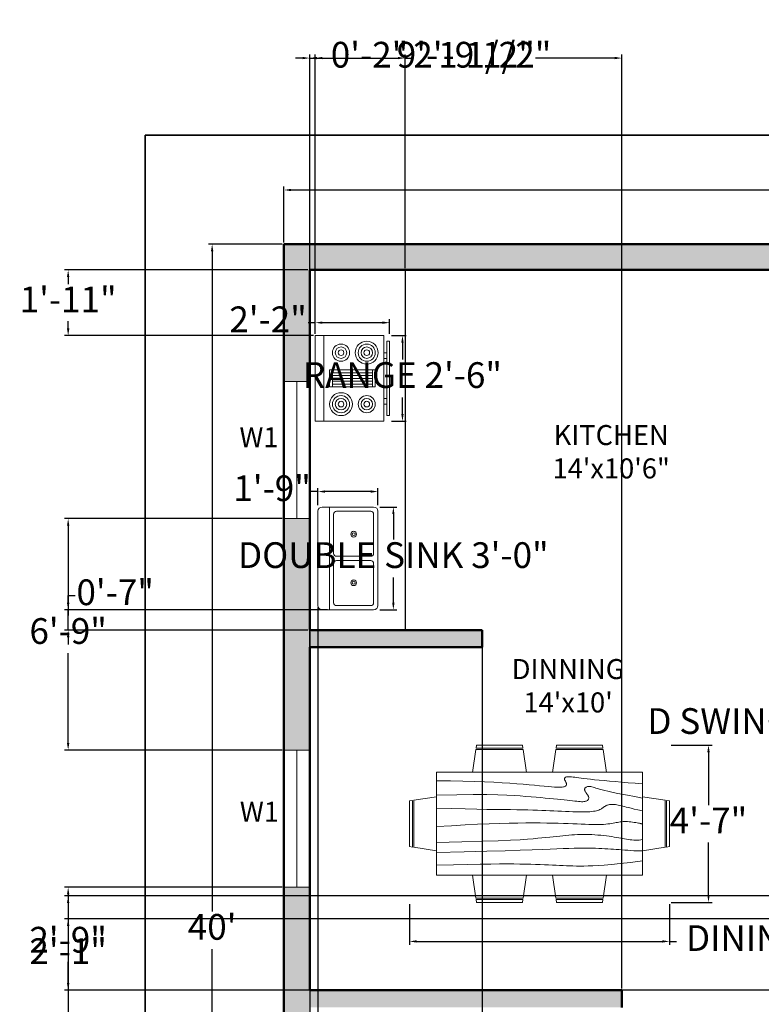
# Model space of a CAD drawing. Units: inches. Extents: x 6193 to 6719, y 6945 to 7563.
# Tile 3 of 4: x 6200 to 6459, y 7219 to 7563. Entities that reach past the tile are written whole.
import ezdxf

# ---------------------------------------------------------------- set-up
doc = ezdxf.new("R2010")
doc.units = ezdxf.units.IN
for name, color, linetype, lineweight in [('A-ANNO-DIMS', 2, 'Continuous', 18), ('A-ANNO-TEXT', 7, 'Continuous', 18), ('A-ANNO-TTLB', 7, 'Continuous', 35), ('A-AREA-IDEN', 7, 'Continuous', 25), ('A-EQPM', 8, 'Continuous', 18), ('A-FLOR-CASE', 8, 'Continuous', 25), ('A-FLOR-FIXT', 9, 'Continuous', 18), ('A-FURN', 8, 'Continuous', 18), ('A-GLAZ', 4, 'Continuous', 18), ('A-WALL', 7, 'Continuous', 50)]:
    doc.layers.add(name, color=color, linetype=linetype, lineweight=lineweight)
doc.layers.add('A-WALL-PATT', color=18, linetype='Continuous', lineweight=13, true_color=0x000000)
doc.styles.get("Standard").update_dxf_attribs({"font": 'arial.ttf'})
doc.dimstyles.new('ISO-25', dxfattribs={"dimtxt": 9, "dimasz": 2.5, "dimexe": 1.25, "dimexo": 0.625, "dimgap": 2, "dimtad": 0, "dimtih": 1, "dimtoh": 1, "dimdec": 1, "dimlunit": 4, "dimtxsty": 'Standard', "dimcen": 2.5, "dimadec": 0, "dimazin": 0, "dimtfac": 0.5, "dimtdec": 1, "dimtmove": 0, "dimatfit": 3, "dimfxl": 1, "dimarcsym": 0})

# ---------------------------------------------------------------- blocks, each defined once
blk = doc.blocks.new('Dining Set - 36 x 72 in.')
for p, q in [((-22.2343, 26.00059), (-23.4847, 17.99762)), ((-22.2304, 26), (-5.7608, 26)), ((-22, 27.5), (-22.1562, 26.50042)), ((-5.8416, 26.5), (-22.1534, 26.5)), ((-22, 27.5), (-6, 27.5)), ((-5.8437, 26.49966), (-6, 27.5)), ((-4.5152, 17.99762), (-5.7655, 25.99926)), ((5.7657, 26.00059), (4.5153, 17.99762)), ((5.7696, 26), (22.2392, 26)), ((6, 27.5), (5.8438, 26.50042)), ((22.1584, 26.5), (5.8466, 26.5)), ((6, 27.5), (22, 27.5)), ((22.1563, 26.49966), (22, 27.5)), ((23.4848, 17.99762), (22.2345, 25.99926)), ((36, 18), (-36, 18)), ((-36, 18), (-36, -18)), ((36, -18), (36, 18)), ((-45.5, 8), (-44.5004, 8.15617)), ((-45.5, 8), (-45.5, -8)), ((-44.5, -8.15843), (-44.5, 8.15338)), ((-44.0006, 8.23428), (-35.9976, 9.48474)), ((-44, 8.23041), (-44, -8.23915)), ((44.0006, 8.23428), (35.9976, 9.48474)), ((44, 8.23041), (44, -8.23915)), ((44.5, -8.15843), (44.5, 8.15338)), ((45.5, 8), (44.5005, 8.15617)), ((45.5, 8), (45.5, -8)), ((-44.4997, -8.15631), (-45.5, -8)), ((-35.9976, -9.48476), (-43.9993, -8.2345)), ((35.9976, -9.48476), (43.9993, -8.2345)), ((44.4997, -8.15631), (45.5, -8)), ((-36, -18), (36, -18)), ((-22.2343, -26.0006), (-23.4847, -17.99762)), ((-4.5152, -17.99762), (-5.7655, -25.99928)), ((5.7657, -26.0006), (4.5153, -17.99762)), ((23.4848, -17.99762), (22.2345, -25.99928)), ((-22.2304, -26), (-5.7608, -26)), ((-22, -27.5), (-22.1562, -26.50044)), ((-5.8416, -26.5), (-22.1534, -26.5)), ((-22, -27.5), (-6, -27.5)), ((-5.8437, -26.49967), (-6, -27.5)), ((5.7696, -26), (22.2392, -26)), ((6, -27.5), (5.8438, -26.50044)), ((22.1584, -26.5), (5.8466, -26.5)), ((6, -27.5), (22, -27.5)), ((22.1563, -26.49967), (22, -27.5))]:
    blk.add_line(p, q)
for points in [[(-36, 15), (-31.1772, 14.97754), (-26.8079, 14.91406), (-22.8538, 14.81543), (-19.276, 14.6875), (-16.0362, 14.53613), (-13.0957, 14.36718), (-10.4159, 14.18652), (-7.9583, 14), (-5.6904, 13.81315), (-3.6035, 13.63021), (-1.6954, 13.45508), (0.0365, 13.29166), (1.5945, 13.14388), (2.9811, 13.01562), (4.1988, 12.9108), (5.25, 12.83333), (6.1393, 12.78613), (6.8802, 12.76823), (7.4883, 12.77767), (7.9792, 12.8125), (8.3685, 12.87077), (8.6719, 12.95052), (8.9049, 13.0498), (9.0833, 13.16666), (9.2205, 13.29899), (9.3216, 13.44401), (9.3895, 13.59879), (9.4271, 13.76041), (9.4373, 13.92594), (9.4232, 14.09245), (9.3875, 14.257), (9.3333, 14.41666), (9.2638, 14.56917), (9.1836, 14.71484), (9.0975, 14.85465), (9.0104, 14.98958), (8.9272, 15.1206), (8.8529, 15.2487), (8.7922, 15.37483), (8.75, 15.5), (8.7305, 15.62467), (8.7344, 15.74739), (8.7617, 15.86621), (8.8125, 15.97916), (8.8867, 16.08431), (8.9844, 16.17968), (9.1055, 16.26334), (9.25, 16.33333), (9.4189, 16.38802), (9.6172, 16.42708), (9.8506, 16.45052), (10.125, 16.45833), (10.4463, 16.45052), (10.8203, 16.42708), (11.2529, 16.38802), (11.75, 16.33333), (12.3184, 16.26318), (12.9694, 16.17838), (13.7151, 16.07991), (14.5677, 15.96875), (15.5395, 15.84586), (16.6426, 15.71224), (17.8893, 15.56884), (19.2917, 15.41666), (20.859, 15.25667), (22.5879, 15.08984), (24.4721, 14.91715), (26.5052, 14.73958), (28.6809, 14.5581), (30.9929, 14.3737), (33.4347, 14.18733), (36, 14)], [(-36, 10), (-28.9766, 10.14274), (-23.1725, 10.20442), (-18.4241, 10.19775), (-14.5677, 10.13541), (-11.4399, 10.03011), (-8.877, 9.89453), (-6.7154, 9.74137), (-4.7917, 9.58333), (-2.9698, 9.43082), (-1.2246, 9.28515), (0.4415, 9.14534), (2.026, 9.01041), (3.5266, 8.87939), (4.9408, 8.7513), (6.266, 8.62516), (7.5, 8.5), (8.6411, 8.37549), (9.6914, 8.2539), (10.6538, 8.13818), (11.5312, 8.03125), (12.3267, 7.93603), (13.043, 7.85547), (13.6831, 7.79248), (14.25, 7.75), (14.7471, 7.7303), (15.1797, 7.73307), (15.5537, 7.75732), (15.875, 7.80208), (16.1494, 7.86637), (16.3828, 7.94922), (16.5811, 8.04964), (16.75, 8.16666), (16.8944, 8.29915), (17.0143, 8.44531), (17.1089, 8.60319), (17.1771, 8.77083), (17.218, 8.94629), (17.2305, 9.1276), (17.2137, 9.31282), (17.1667, 9.5), (17.0895, 9.6875), (16.987, 9.875), (16.8649, 10.0625), (16.7292, 10.25), (16.5856, 10.4375), (16.4401, 10.625), (16.2985, 10.8125), (16.1667, 11), (16.05, 11.18733), (15.9518, 11.3737), (15.8752, 11.5581), (15.8229, 11.73958), (15.798, 11.91715), (15.8034, 12.08984), (15.842, 12.25667), (15.9167, 12.41666), (16.0295, 12.56836), (16.1784, 12.70833), (16.3605, 12.83268), (16.5729, 12.9375), (16.8127, 13.01888), (17.0768, 13.07291), (17.3625, 13.0957), (17.6667, 13.08333), (17.9894, 13.03312), (18.3418, 12.94726), (18.7382, 12.82918), (19.1927, 12.68229), (19.7195, 12.51001), (20.3327, 12.31575), (21.0465, 12.10294), (21.875, 11.875), (22.8357, 11.63354), (23.959, 11.37304), (25.2786, 11.08618), (26.8282, 10.76562), (28.6414, 10.40405), (30.752, 9.99414), (33.1936, 9.52856), (36, 9)], [(-36, 5.5), (-30.7157, 5.3348), (-26.069, 5.20963), (-21.9946, 5.11767), (-18.4271, 5.05208), (-15.3009, 5.00602), (-12.5508, 4.97265), (-10.1112, 4.94515), (-7.9167, 4.91666), (-5.909, 4.88167), (-4.0586, 4.83984), (-2.3429, 4.79215), (-0.7396, 4.73958), (0.7739, 4.6831), (2.22, 4.6237), (3.6213, 4.56233), (5, 4.5), (6.373, 4.43782), (7.7344, 4.3776), (9.0723, 4.32129), (10.375, 4.27083), (11.6309, 4.22819), (12.8281, 4.19531), (13.9551, 4.17415), (15, 4.16666), (15.954, 4.17448), (16.819, 4.19791), (17.6001, 4.23698), (18.3021, 4.29166), (18.9299, 4.36198), (19.4883, 4.44791), (19.9823, 4.54948), (20.4167, 4.66666), (20.7969, 4.79899), (21.1302, 4.94401), (21.4245, 5.09879), (21.6875, 5.26041), (21.9271, 5.42594), (22.1511, 5.59245), (22.3672, 5.757), (22.5834, 5.91666), (22.8065, 6.06868), (23.0404, 6.21093), (23.2879, 6.34147), (23.5521, 6.45833), (23.8358, 6.55957), (24.142, 6.64323), (24.4735, 6.70735), (24.8334, 6.75), (25.2235, 6.76969), (25.642, 6.76692), (26.0858, 6.74267), (26.5521, 6.69791), (27.0379, 6.63362), (27.5404, 6.55078), (28.0565, 6.45036), (28.5834, 6.33333), (29.1242, 6.19987), (29.7071, 6.04687), (30.3661, 5.87044), (31.1354, 5.66666), (32.0493, 5.43164), (33.142, 5.16146), (34.4475, 4.85221), (36, 4.5)], [(-36, -1), (-30.7915, -0.6591), (-26.0195, -0.38216), (-21.6519, -0.16284), (-17.6563, 0.00521), (-14.0005, 0.12833), (-10.6523, 0.21289), (-7.5796, 0.26522), (-4.75, 0.29166), (-2.134, 0.29793), (0.2878, 0.28711), (2.5317, 0.26163), (4.6146, 0.22396), (6.5529, 0.17651), (8.3633, 0.12174), (10.0623, 0.06209), (11.6667, 0), (13.1899, -0.06201), (14.6341, -0.1211), (15.9982, -0.17432), (17.2813, -0.21875), (18.4823, -0.25147), (19.6003, -0.26953), (20.6343, -0.27002), (21.5834, -0.25), (22.4481, -0.20768), (23.2357, -0.14584), (23.9549, -0.06836), (24.6146, 0.02083), (25.2235, 0.11784), (25.7904, 0.21875), (26.3241, 0.31966), (26.8334, 0.41666), (27.3265, 0.50618), (27.8099, 0.58593), (28.2894, 0.65397), (28.7709, 0.70833), (29.2601, 0.74707), (29.763, 0.76823), (30.2855, 0.76985), (30.8334, 0.75), (31.4088, 0.70784), (31.9994, 0.64713), (32.589, 0.57275), (33.1615, 0.48958), (33.7008, 0.4025), (34.1908, 0.3164), (34.6153, 0.23616), (34.9584, 0.16666), (35.2099, 0.11165), (35.3848, 0.07031), (35.504, 0.04069), (35.5886, 0.02083), (35.6594, 0.00879), (35.7377, 0.0026), (35.8442, 0.00032), (36, 0)], [(-36, -6.5), (-27.1843, -6.31267), (-20.084, -6.1263), (-14.469, -5.9419), (-10.1094, -5.76042), (-6.7752, -5.58285), (-4.2363, -5.41016), (-2.2629, -5.24333), (-0.625, -5.08334), (0.8708, -4.93099), (2.2715, -4.78646), (3.5872, -4.64974), (4.8281, -4.52084), (6.0046, -4.39974), (7.127, -4.28646), (8.2053, -4.18099), (9.25, -4.08334), (10.2705, -3.99382), (11.2734, -3.91407), (12.2647, -3.84603), (13.25, -3.79167), (14.2354, -3.75293), (15.2266, -3.73177), (16.2295, -3.73015), (17.25, -3.75), (18.2912, -3.79248), (19.3451, -3.85547), (20.4009, -3.93604), (21.4479, -4.03125), (22.4754, -4.13819), (23.4727, -4.25391), (24.4289, -4.37549), (25.3334, -4.5), (26.1785, -4.62492), (26.9694, -4.74935), (27.7145, -4.87281), (28.4219, -4.99479), (29.1, -5.11483), (29.7572, -5.23242), (30.4016, -5.34709), (31.0417, -5.45834), (31.6837, -5.56437), (32.3262, -5.65821), (32.9658, -5.73153), (33.599, -5.77604), (34.2224, -5.78345), (34.8327, -5.74545), (35.4264, -5.65373), (36, -5.5)], [(-36, -10), (-26.4022, -9.81299), (-18.4675, -9.62891), (-11.9839, -9.45069), (-6.7396, -9.28125), (-2.5226, -9.12354), (0.8789, -8.98047), (3.6769, -8.85498), (6.0833, -8.75), (8.2767, -8.66765), (10.3021, -8.60677), (12.1712, -8.56543), (13.8958, -8.54167), (15.4876, -8.53353), (16.9583, -8.53907), (18.3197, -8.55632), (19.5834, -8.58334), (20.7616, -8.61841), (21.8685, -8.66081), (22.9188, -8.71004), (23.9271, -8.76563), (24.9081, -8.82707), (25.8763, -8.89388), (26.8465, -8.96558), (27.8334, -9.04167), (28.8474, -9.12118), (29.8828, -9.20117), (30.93, -9.27824), (31.9792, -9.34896), (33.0205, -9.40991), (34.0443, -9.45768), (35.0407, -9.48885), (36, -9.5)], [(-36, -14.5), (-30.0881, -14.33513), (-25.0332, -14.21224), (-20.7312, -14.12647), (-17.0781, -14.07292), (-13.97, -14.04671), (-11.3027, -14.04297), (-8.9724, -14.05681), (-6.875, -14.08334), (-4.9224, -14.11833), (-3.0905, -14.16016), (-1.3709, -14.20785), (0.2448, -14.26042), (1.7647, -14.3169), (3.1973, -14.3763), (4.5507, -14.43767), (5.8333, -14.5), (7.0554, -14.5621), (8.235, -14.62175), (9.3922, -14.67652), (10.5469, -14.72396), (11.7192, -14.76164), (12.929, -14.78711), (14.1965, -14.79794), (15.5417, -14.79167), (16.9933, -14.76424), (18.6152, -14.70508), (20.4804, -14.60197), (22.6615, -14.44271), (25.2312, -14.21509), (28.2624, -13.9069), (31.8277, -13.50594), (36, -13)]]:
    blk.add_lwpolyline(points)
blk = doc.blocks.new('Range-Oven - 30 in top')
for p, q in [((0, -3), (30, -3)), ((12, -6), (18, -6)), ((13, -20), (13, -6)), ((14, -6), (14, -20)), ((15, -20), (15, -6)), ((16, -6), (16, -20)), ((17, -20), (17, -6)), ((18, -20), (12, -20)), ((6, -24), (6, -25)), ((8, -25), (8, -24)), ((22, -25), (22, -24)), ((24, -24), (24, -25))]:
    blk.add_line(p, q)
for points in [[(0, -24), (0, 0), (30, 0), (30, -24)], [(12, -21), (12, -5), (18, -5), (18, -21)], [(2, -26), (2, -25), (28, -25), (28, -26)]]:
    blk.add_lwpolyline(points, close=True)
for centre, radius in [((6, -9), 4), ((6, -9), 3), ((24, -9), 3), ((6, -9), 2), ((6, -9), 1), ((24, -9), 2), ((24, -9), 1), ((6, -18), 3), ((6, -18), 2), ((6, -18), 1), ((24, -18), 4), ((24, -18), 3), ((24, -18), 2), ((24, -18), 1)]:
    blk.add_circle(centre, radius)
blk = doc.blocks.new('Sink-double - 36 in top')
for p, q in [((-18, -4), (18, -4)), ((-0.75, -18.5), (-0.75, -6.5)), ((0.75, -6.5), (0.75, -18.5))]:
    blk.add_line(p, q)
for points in [[(-16.5, 0), (16.5, 0)], [(-18, -19.5), (-18, -1.5)], [(18, -1.5), (18, -19.5)], [(-16.5, -18.5), (-16.5, -6.5)], [(-15.5, -5.5), (-1.75, -5.5)], [(1.75, -5.5), (15.5, -5.5)], [(16.5, -6.5), (16.5, -18.5)], [(-1.75, -19.5), (-15.5, -19.5)], [(15.5, -19.5), (1.75, -19.5)], [(16.5, -21), (-16.5, -21)]]:
    blk.add_lwpolyline(points)
for centre, radius in [((-8.5, -12.5), 1), ((-8.5, -12.5), 0.5), ((8.5, -12.5), 1), ((8.5, -12.5), 0.5)]:
    blk.add_circle(centre, radius)
for centre, radius, start, end in [((-16.5, -1.5), 1.5, 90, 180), ((16.5, -1.5), 1.5, 0, 90), ((-15.5, -6.5), 1, 90, 180), ((-1.75, -6.5), 1, 0, 90), ((1.75, -6.5), 1, 90, 180), ((15.5, -6.5), 1, 0, 90), ((-16.5, -19.5), 1.5, 180, 270), ((-15.5, -18.5), 1, 180, 270), ((-1.75, -18.5), 1, 270, 0), ((1.75, -18.5), 1, 180, 270), ((15.5, -18.5), 1, 270, 0), ((16.5, -19.5), 1.5, 270, 0)]:
    blk.add_arc(centre, radius, start, end)
blk = doc.blocks.new('*D10')
at = {"layer": 'A-ANNO-DIMS', "color": 0, "lineweight": -2, "transparency": 16777216}
for p, q in [((6292.28, 7485.29), (6292.28, 7504.87)), ((6294.78, 7503.62), (6462.65, 7503.62)), ((6649.78, 7503.62), (6481.92, 7503.62)), ((6652.28, 7485.29), (6652.28, 7504.87))]:
    blk.add_line(p, q, dxfattribs=at)
at = {"layer": 'A-ANNO-DIMS', "color": 0, "transparency": 16777216}
for points in [[(6294.78, 7504.03), (6294.78, 7503.2), (6292.28, 7503.62)], [(6649.78, 7504.03), (6649.78, 7503.2), (6652.28, 7503.62)]]:
    blk.add_solid(points, dxfattribs=at)
at = {"layer": 'Defpoints', "color": 0, "transparency": 16777216}
for p in [(6652.28, 7503.62), (6292.28, 7484.66), (6652.28, 7484.66)]:
    blk.add_point(p, dxfattribs=at)
at = {"layer": 'A-ANNO-DIMS', "color": 0, "transparency": 16777216, "insert": (6472.28, 7503.62), "char_height": 9, "attachment_point": 5}
blk.add_mtext("30'", dxfattribs=at)
blk = doc.blocks.new('*D11')
at = {"layer": 'A-ANNO-DIMS', "color": 0, "lineweight": -2, "transparency": 16777216}
for p, q in [((6291.66, 7484.66), (6265.88, 7484.66)), ((6267.13, 7482.16), (6267.13, 7251.26)), ((6267.13, 7007.16), (6267.13, 7238.07)), ((6291.66, 7004.66), (6265.88, 7004.66))]:
    blk.add_line(p, q, dxfattribs=at)
at = {"layer": 'A-ANNO-DIMS', "color": 0, "transparency": 16777216}
for points in [[(6266.71, 7482.16), (6267.55, 7482.16), (6267.13, 7484.66)], [(6266.71, 7007.16), (6267.55, 7007.16), (6267.13, 7004.66)]]:
    blk.add_solid(points, dxfattribs=at)
at = {"layer": 'Defpoints', "color": 0, "transparency": 16777216}
for p in [(6292.28, 7484.66), (6267.13, 7004.66), (6292.28, 7004.66)]:
    blk.add_point(p, dxfattribs=at)
at = {"layer": 'A-ANNO-DIMS', "color": 0, "transparency": 16777216, "insert": (6267.13, 7244.66), "char_height": 9, "attachment_point": 5}
blk.add_mtext("40'", dxfattribs=at)
blk = doc.blocks.new('WIN-48IN')
for p, q in [((0, 48), (9, 48)), ((4.5, 48), (4.5, 0)), ((0, 0), (9, 0))]:
    blk.add_line(p, q)
blk = doc.blocks.new('*D20')
at = {"layer": 'A-ANNO-DIMS', "color": 0, "lineweight": -2, "transparency": 16777216}
for p, q in [((6479.1, 7337.66), (6472.18, 7337.66)), ((6473.43, 7335.16), (6473.43, 7323.32)), ((6473.43, 7298.16), (6473.43, 7310.01)), ((6479.1, 7295.66), (6472.18, 7295.66))]:
    blk.add_line(p, q, dxfattribs=at)
at = {"layer": 'A-ANNO-DIMS', "color": 0, "transparency": 16777216}
for points in [[(6473.01, 7335.16), (6473.84, 7335.16), (6473.43, 7337.66)], [(6473.01, 7298.16), (6473.84, 7298.16), (6473.43, 7295.66)]]:
    blk.add_solid(points, dxfattribs=at)
at = {"layer": 'Defpoints', "color": 0, "transparency": 16777216}
for p in [(6473.43, 7337.66), (6479.73, 7337.66), (6479.73, 7295.66)]:
    blk.add_point(p, dxfattribs=at)
at = {"layer": 'A-ANNO-DIMS', "color": 0, "transparency": 16777216, "insert": (6473.43, 7316.66), "char_height": 9, "attachment_point": 5}
blk.add_mtext('D SWING 3\'-6" TYP.', dxfattribs=at)
blk = doc.blocks.new('*D22')
at = {"layer": 'A-ANNO-DIMS', "color": 0, "lineweight": -2, "transparency": 16777216}
for p, q in [((6336.22, 7253.77), (6336.22, 7239.49)), ((6427.22, 7253.77), (6427.22, 7239.49)), ((6338.72, 7240.74), (6424.72, 7240.74)), ((6427.22, 7240.74), (6429.72, 7240.74))]:
    blk.add_line(p, q, dxfattribs=at)
at = {"layer": 'A-ANNO-DIMS', "color": 0, "transparency": 16777216}
for points in [[(6338.72, 7241.16), (6338.72, 7240.33), (6336.22, 7240.74)], [(6424.72, 7241.16), (6424.72, 7240.33), (6427.22, 7240.74)]]:
    blk.add_solid(points, dxfattribs=at)
at = {"layer": 'Defpoints', "color": 0, "transparency": 16777216}
for p in [(6336.22, 7254.39), (6427.22, 7254.39), (6427.22, 7240.74)]:
    blk.add_point(p, dxfattribs=at)
at = {"layer": 'A-ANNO-DIMS', "color": 0, "transparency": 16777216, "insert": (6481.18, 7240.74), "char_height": 9, "attachment_point": 5}
blk.add_mtext('DINING SET 7\'-7"', dxfattribs=at)
blk = doc.blocks.new('*D23')
at = {"layer": 'A-ANNO-DIMS', "color": 0, "lineweight": -2, "transparency": 16777216}
for p, q in [((6427.84, 7309.39), (6442.12, 7309.39)), ((6440.87, 7306.89), (6440.87, 7288.39)), ((6440.87, 7256.89), (6440.87, 7275.39)), ((6427.84, 7254.39), (6442.12, 7254.39))]:
    blk.add_line(p, q, dxfattribs=at)
at = {"layer": 'A-ANNO-DIMS', "color": 0, "transparency": 16777216}
for points in [[(6440.45, 7306.89), (6441.29, 7306.89), (6440.87, 7309.39)], [(6440.45, 7256.89), (6441.29, 7256.89), (6440.87, 7254.39)]]:
    blk.add_solid(points, dxfattribs=at)
at = {"layer": 'Defpoints', "color": 0, "transparency": 16777216}
for p in [(6427.22, 7309.39), (6440.87, 7309.39), (6427.22, 7254.39)]:
    blk.add_point(p, dxfattribs=at)
at = {"layer": 'A-ANNO-DIMS', "color": 0, "transparency": 16777216, "insert": (6440.87, 7281.89), "char_height": 9, "attachment_point": 5}
blk.add_mtext('4\'-7"', dxfattribs=at)
blk = doc.blocks.new('*D30')
at = {"layer": 'A-ANNO-DIMS', "color": 0, "lineweight": -2, "transparency": 16777216}
for p, q in [((6329.88, 7452.7), (6335, 7452.7)), ((6333.75, 7450.2), (6333.75, 7444.36)), ((6333.75, 7425.2), (6333.75, 7431.05)), ((6329.88, 7422.7), (6335, 7422.7))]:
    blk.add_line(p, q, dxfattribs=at)
at = {"layer": 'A-ANNO-DIMS', "color": 0, "transparency": 16777216}
for points in [[(6333.34, 7450.2), (6334.17, 7450.2), (6333.75, 7452.7)], [(6333.34, 7425.2), (6334.17, 7425.2), (6333.75, 7422.7)]]:
    blk.add_solid(points, dxfattribs=at)
at = {"layer": 'Defpoints', "color": 0, "transparency": 16777216}
for p in [(6329.25, 7452.7), (6333.75, 7452.7), (6329.25, 7422.7)]:
    blk.add_point(p, dxfattribs=at)
at = {"layer": 'A-ANNO-DIMS', "color": 0, "transparency": 16777216, "insert": (6333.75, 7437.7), "char_height": 9, "attachment_point": 5}
blk.add_mtext('RANGE 2\'-6"', dxfattribs=at)
blk = doc.blocks.new('*D31')
at = {"layer": 'A-ANNO-DIMS', "color": 0, "lineweight": -2, "transparency": 16777216}
for p, q in [((6303.25, 7453.33), (6303.25, 7458.45)), ((6329.25, 7453.33), (6329.25, 7458.45)), ((6303.25, 7457.2), (6300.75, 7457.2)), ((6326.75, 7457.2), (6305.75, 7457.2))]:
    blk.add_line(p, q, dxfattribs=at)
at = {"layer": 'A-ANNO-DIMS', "color": 0, "transparency": 16777216}
for points in [[(6305.75, 7457.62), (6305.75, 7456.79), (6303.25, 7457.2)], [(6326.75, 7457.62), (6326.75, 7456.79), (6329.25, 7457.2)]]:
    blk.add_solid(points, dxfattribs=at)
at = {"layer": 'Defpoints', "color": 0, "transparency": 16777216}
for p in [(6303.25, 7457.2), (6303.25, 7452.7), (6329.25, 7452.7)]:
    blk.add_point(p, dxfattribs=at)
at = {"layer": 'A-ANNO-DIMS', "color": 0, "transparency": 16777216, "insert": (6286.72, 7457.2), "char_height": 9, "attachment_point": 5}
blk.add_mtext('2\'-2"', dxfattribs=at)
blk = doc.blocks.new('*D32')
at = {"layer": 'A-ANNO-DIMS', "color": 0, "lineweight": -2, "transparency": 16777216}
for p, q in [((6325.79, 7392.71), (6331.82, 7392.71)), ((6330.57, 7390.21), (6330.57, 7381.37)), ((6330.57, 7359.21), (6330.57, 7368.06)), ((6325.79, 7356.71), (6331.82, 7356.71))]:
    blk.add_line(p, q, dxfattribs=at)
at = {"layer": 'A-ANNO-DIMS', "color": 0, "transparency": 16777216}
for points in [[(6330.15, 7390.21), (6330.98, 7390.21), (6330.57, 7392.71)], [(6330.15, 7359.21), (6330.98, 7359.21), (6330.57, 7356.71)]]:
    blk.add_solid(points, dxfattribs=at)
at = {"layer": 'Defpoints', "color": 0, "transparency": 16777216}
for p in [(6325.17, 7392.71), (6330.57, 7392.71), (6325.17, 7356.71)]:
    blk.add_point(p, dxfattribs=at)
at = {"layer": 'A-ANNO-DIMS', "color": 0, "transparency": 16777216, "insert": (6330.57, 7374.71), "char_height": 9, "attachment_point": 5}
blk.add_mtext('DOUBLE SINK 3\'-0"', dxfattribs=at)
blk = doc.blocks.new('*D33')
at = {"layer": 'A-ANNO-DIMS', "color": 0, "lineweight": -2, "transparency": 16777216}
for p, q in [((6304.17, 7393.34), (6304.17, 7399.36)), ((6325.17, 7393.34), (6325.17, 7399.36)), ((6304.17, 7398.11), (6301.67, 7398.11)), ((6322.67, 7398.11), (6306.67, 7398.11))]:
    blk.add_line(p, q, dxfattribs=at)
at = {"layer": 'A-ANNO-DIMS', "color": 0, "transparency": 16777216}
for points in [[(6306.67, 7398.53), (6306.67, 7397.7), (6304.17, 7398.11)], [(6322.67, 7398.53), (6322.67, 7397.7), (6325.17, 7398.11)]]:
    blk.add_solid(points, dxfattribs=at)
at = {"layer": 'Defpoints', "color": 0, "transparency": 16777216}
for p in [(6304.17, 7398.11), (6304.17, 7392.71), (6325.17, 7392.71)]:
    blk.add_point(p, dxfattribs=at)
at = {"layer": 'A-ANNO-DIMS', "color": 0, "transparency": 16777216, "insert": (6288.13, 7398.11), "char_height": 9, "attachment_point": 5}
blk.add_mtext('1\'-9"', dxfattribs=at)
blk = doc.blocks.new('*D35')
at = {"layer": 'A-ANNO-DIMS', "color": 0, "lineweight": -2, "transparency": 16777216}
for p, q in [((6291.66, 7259.66), (6215.49, 7259.66)), ((6216.74, 7257.16), (6216.74, 7206.26)), ((6216.74, 7142.16), (6216.74, 7193.07)), ((6291.66, 7139.66), (6215.49, 7139.66))]:
    blk.add_line(p, q, dxfattribs=at)
at = {"layer": 'A-ANNO-DIMS', "color": 0, "transparency": 16777216}
for points in [[(6216.32, 7257.16), (6217.16, 7257.16), (6216.74, 7259.66)], [(6216.32, 7142.16), (6217.16, 7142.16), (6216.74, 7139.66)]]:
    blk.add_solid(points, dxfattribs=at)
at = {"layer": 'Defpoints', "color": 0, "transparency": 16777216}
for p in [(6216.74, 7259.66), (6292.28, 7259.66), (6292.28, 7139.66)]:
    blk.add_point(p, dxfattribs=at)
at = {"layer": 'A-ANNO-DIMS', "color": 0, "transparency": 16777216, "insert": (6216.74, 7199.66), "char_height": 9, "attachment_point": 5}
blk.add_mtext('10\'-0"', dxfattribs=at)
blk = doc.blocks.new('*D36')
at = {"layer": 'A-ANNO-DIMS', "color": 0, "lineweight": -2, "transparency": 16777216}
for p, q in [((6291.66, 7388.66), (6215.49, 7388.66)), ((6216.74, 7386.16), (6216.74, 7354.76)), ((6216.74, 7310.16), (6216.74, 7341.57)), ((6291.66, 7307.66), (6215.49, 7307.66))]:
    blk.add_line(p, q, dxfattribs=at)
at = {"layer": 'A-ANNO-DIMS', "color": 0, "transparency": 16777216}
for points in [[(6216.32, 7386.16), (6217.16, 7386.16), (6216.74, 7388.66)], [(6216.32, 7310.16), (6217.16, 7310.16), (6216.74, 7307.66)]]:
    blk.add_solid(points, dxfattribs=at)
at = {"layer": 'Defpoints', "color": 0, "transparency": 16777216}
for p in [(6216.74, 7388.66), (6292.28, 7388.66), (6292.28, 7307.66)]:
    blk.add_point(p, dxfattribs=at)
at = {"layer": 'A-ANNO-DIMS', "color": 0, "transparency": 16777216, "insert": (6216.74, 7348.16), "char_height": 9, "attachment_point": 5}
blk.add_mtext('6\'-9"', dxfattribs=at)
blk = doc.blocks.new('*D53')
at = {"layer": 'A-ANNO-DIMS', "color": 0, "lineweight": -2, "transparency": 16777216}
for p, q in [((6564.66, 7248.66), (6215.49, 7248.66)), ((6216.74, 7246.16), (6216.74, 7242.68)), ((6216.74, 7226.16), (6216.74, 7229.64)), ((6564.66, 7223.66), (6215.49, 7223.66))]:
    blk.add_line(p, q, dxfattribs=at)
at = {"layer": 'A-ANNO-DIMS', "color": 0, "transparency": 16777216}
for points in [[(6216.32, 7246.16), (6217.16, 7246.16), (6216.74, 7248.66)], [(6216.32, 7226.16), (6217.16, 7226.16), (6216.74, 7223.66)]]:
    blk.add_solid(points, dxfattribs=at)
at = {"layer": 'Defpoints', "color": 0, "transparency": 16777216}
for p in [(6216.74, 7248.66), (6565.28, 7248.66), (6565.28, 7223.66)]:
    blk.add_point(p, dxfattribs=at)
at = {"layer": 'A-ANNO-DIMS', "color": 0, "transparency": 16777216, "insert": (6216.74, 7236.16), "char_height": 9, "attachment_point": 5}
blk.add_mtext('2\'-1"', dxfattribs=at)
blk = doc.blocks.new('*D55')
at = {"layer": 'A-ANNO-DIMS', "color": 0, "lineweight": -2, "transparency": 16777216}
for p, q in [((6627.43, 7256.66), (6215.49, 7256.66)), ((6216.74, 7254.16), (6216.74, 7246.76)), ((6216.74, 7226.16), (6216.74, 7233.57)), ((6616.93, 7223.66), (6215.49, 7223.66))]:
    blk.add_line(p, q, dxfattribs=at)
at = {"layer": 'A-ANNO-DIMS', "color": 0, "transparency": 16777216}
for points in [[(6216.32, 7254.16), (6217.16, 7254.16), (6216.74, 7256.66)], [(6216.32, 7226.16), (6217.16, 7226.16), (6216.74, 7223.66)]]:
    blk.add_solid(points, dxfattribs=at)
at = {"layer": 'Defpoints', "color": 0, "transparency": 16777216}
for p in [(6216.74, 7256.66), (6628.06, 7256.66), (6617.56, 7223.66)]:
    blk.add_point(p, dxfattribs=at)
at = {"layer": 'A-ANNO-DIMS', "color": 0, "transparency": 16777216, "insert": (6216.74, 7240.16), "char_height": 9, "attachment_point": 5}
blk.add_mtext('2\'-9"', dxfattribs=at)
blk = doc.blocks.new('*D57')
at = {"layer": 'A-ANNO-DIMS', "color": 0, "lineweight": -2, "transparency": 16777216}
for p, q in [((6301.28, 7349.04), (6301.28, 6957.2)), ((6361.63, 7349.04), (6361.63, 6957.2)), ((6303.78, 6958.45), (6307.01, 6958.45)), ((6359.13, 6958.45), (6355.91, 6958.45))]:
    blk.add_line(p, q, dxfattribs=at)
at = {"layer": 'A-ANNO-DIMS', "color": 0, "transparency": 16777216}
for points in [[(6303.78, 6958.86), (6303.78, 6958.03), (6301.28, 6958.45)], [(6359.13, 6958.86), (6359.13, 6958.03), (6361.63, 6958.45)]]:
    blk.add_solid(points, dxfattribs=at)
at = {"layer": 'Defpoints', "color": 0, "transparency": 16777216}
for p in [(6301.28, 7349.66), (6361.63, 7349.66), (6361.63, 6958.45)]:
    blk.add_point(p, dxfattribs=at)
at = {"layer": 'A-ANNO-DIMS', "color": 0, "transparency": 16777216, "insert": (6331.46, 6958.45), "char_height": 9, "attachment_point": 5}
blk.add_mtext('5\'-0 1/2"', dxfattribs=at)
blk = doc.blocks.new('*D58')
at = {"layer": 'A-ANNO-DIMS', "color": 0, "lineweight": -2, "transparency": 16777216}
for p, q in [((6301.28, 7476.29), (6301.28, 7551.02)), ((6334.69, 7476.29), (6334.69, 7551.02)), ((6303.78, 7549.77), (6332.19, 7549.77)), ((6334.69, 7549.77), (6337.19, 7549.77))]:
    blk.add_line(p, q, dxfattribs=at)
at = {"layer": 'A-ANNO-DIMS', "color": 0, "transparency": 16777216}
for points in [[(6303.78, 7550.19), (6303.78, 7549.36), (6301.28, 7549.77)], [(6332.19, 7550.19), (6332.19, 7549.36), (6334.69, 7549.77)]]:
    blk.add_solid(points, dxfattribs=at)
at = {"layer": 'Defpoints', "color": 0, "transparency": 16777216}
for p in [(6334.69, 7549.77), (6301.28, 7475.66), (6334.69, 7475.66)]:
    blk.add_point(p, dxfattribs=at)
at = {"layer": 'A-ANNO-DIMS', "color": 0, "transparency": 16777216, "insert": (6361.72, 7549.77), "char_height": 9, "attachment_point": 5}
blk.add_mtext('2\'-9 1/2"', dxfattribs=at)
blk = doc.blocks.new('*D59')
at = {"layer": 'A-ANNO-DIMS', "color": 0, "lineweight": -2, "transparency": 16777216}
for p, q in [((6300.66, 7475.66), (6215.49, 7475.66)), ((6216.74, 7473.16), (6216.74, 7470.7)), ((6216.74, 7455.2), (6216.74, 7457.67)), ((6302.63, 7452.7), (6215.49, 7452.7))]:
    blk.add_line(p, q, dxfattribs=at)
at = {"layer": 'A-ANNO-DIMS', "color": 0, "transparency": 16777216}
for points in [[(6216.32, 7473.16), (6217.16, 7473.16), (6216.74, 7475.66)], [(6216.32, 7455.2), (6217.16, 7455.2), (6216.74, 7452.7)]]:
    blk.add_solid(points, dxfattribs=at)
at = {"layer": 'Defpoints', "color": 0, "transparency": 16777216}
for p in [(6301.28, 7475.66), (6216.74, 7452.7), (6303.25, 7452.7)]:
    blk.add_point(p, dxfattribs=at)
at = {"layer": 'A-ANNO-DIMS', "color": 0, "transparency": 16777216, "insert": (6216.74, 7464.18), "char_height": 9, "attachment_point": 5}
blk.add_mtext('1\'-11"', dxfattribs=at)
blk = doc.blocks.new('*D60')
at = {"layer": 'A-ANNO-DIMS', "color": 0, "lineweight": -2, "transparency": 16777216}
for p, q in [((6216.74, 7359.21), (6216.74, 7361.71)), ((6216.74, 7361.71), (6219.24, 7361.71)), ((6307.54, 7356.71), (6215.49, 7356.71)), ((6216.74, 7349.66), (6216.74, 7356.71)), ((6300.66, 7349.66), (6215.49, 7349.66)), ((6216.74, 7347.16), (6216.74, 7344.66))]:
    blk.add_line(p, q, dxfattribs=at)
at = {"layer": 'A-ANNO-DIMS', "color": 0, "transparency": 16777216}
for points in [[(6216.32, 7359.21), (6217.16, 7359.21), (6216.74, 7356.71)], [(6216.32, 7347.16), (6217.16, 7347.16), (6216.74, 7349.66)]]:
    blk.add_solid(points, dxfattribs=at)
at = {"layer": 'Defpoints', "color": 0, "transparency": 16777216}
for p in [(6216.74, 7356.71), (6308.17, 7356.71), (6301.28, 7349.66)]:
    blk.add_point(p, dxfattribs=at)
at = {"layer": 'A-ANNO-DIMS', "color": 0, "transparency": 16777216, "insert": (6233.2, 7361.71), "char_height": 9, "attachment_point": 5}
blk.add_mtext('0\'-7"', dxfattribs=at)
blk = doc.blocks.new('*D61')
at = {"layer": 'A-ANNO-DIMS', "color": 0, "lineweight": -2, "transparency": 16777216}
for p, q in [((6301.28, 7476.29), (6301.28, 7551.02)), ((6303.25, 7453.33), (6303.25, 7551.02)), ((6298.78, 7549.77), (6296.28, 7549.77)), ((6301.28, 7549.77), (6303.25, 7549.77)), ((6305.75, 7549.77), (6308.25, 7549.77))]:
    blk.add_line(p, q, dxfattribs=at)
at = {"layer": 'A-ANNO-DIMS', "color": 0, "transparency": 16777216}
for points in [[(6298.78, 7550.19), (6298.78, 7549.36), (6301.28, 7549.77)], [(6305.75, 7550.19), (6305.75, 7549.36), (6303.25, 7549.77)]]:
    blk.add_solid(points, dxfattribs=at)
at = {"layer": 'Defpoints', "color": 0, "transparency": 16777216}
for p in [(6303.25, 7549.77), (6301.28, 7475.66), (6303.25, 7452.7)]:
    blk.add_point(p, dxfattribs=at)
at = {"layer": 'A-ANNO-DIMS', "color": 0, "transparency": 16777216, "insert": (6322.22, 7549.77), "char_height": 9, "attachment_point": 5}
blk.add_mtext('0\'-2"', dxfattribs=at)
blk = doc.blocks.new('*D62')
at = {"layer": 'A-ANNO-DIMS', "color": 0, "lineweight": -2, "transparency": 16777216}
for p, q in [((6304.17, 7357.59), (6304.17, 6957.2)), ((6301.28, 7349.04), (6301.28, 6957.2)), ((6298.78, 6958.45), (6296.28, 6958.45)), ((6301.28, 6958.45), (6304.17, 6958.45)), ((6306.67, 6958.45), (6309.17, 6958.45))]:
    blk.add_line(p, q, dxfattribs=at)
at = {"layer": 'A-ANNO-DIMS', "color": 0, "transparency": 16777216}
for points in [[(6298.78, 6958.86), (6298.78, 6958.03), (6301.28, 6958.45)], [(6306.67, 6958.86), (6306.67, 6958.03), (6304.17, 6958.45)]]:
    blk.add_solid(points, dxfattribs=at)
at = {"layer": 'Defpoints', "color": 0, "transparency": 16777216}
for p in [(6304.17, 7358.21), (6301.28, 7349.66), (6304.17, 6958.45)]:
    blk.add_point(p, dxfattribs=at)
at = {"layer": 'A-ANNO-DIMS', "color": 0, "transparency": 16777216, "insert": (6323.13, 6958.45), "char_height": 9, "attachment_point": 5}
blk.add_mtext('0\'-3"', dxfattribs=at)
blk = doc.blocks.new('*D63')
at = {"layer": 'A-ANNO-DIMS', "color": 0, "lineweight": -2, "transparency": 16777216}
for p, q in [((6301.28, 7224.29), (6301.28, 7551.02)), ((6410.54, 7224.29), (6410.54, 7551.02)), ((6303.78, 7549.77), (6331.47, 7549.77)), ((6408.04, 7549.77), (6380.36, 7549.77))]:
    blk.add_line(p, q, dxfattribs=at)
at = {"layer": 'A-ANNO-DIMS', "color": 0, "transparency": 16777216}
for points in [[(6303.78, 7550.19), (6303.78, 7549.36), (6301.28, 7549.77)], [(6408.04, 7550.19), (6408.04, 7549.36), (6410.54, 7549.77)]]:
    blk.add_solid(points, dxfattribs=at)
at = {"layer": 'Defpoints', "color": 0, "transparency": 16777216}
for p in [(6410.54, 7549.77), (6301.28, 7223.66), (6410.54, 7223.66)]:
    blk.add_point(p, dxfattribs=at)
at = {"layer": 'A-ANNO-DIMS', "color": 0, "transparency": 16777216, "insert": (6355.91, 7549.77), "char_height": 9, "attachment_point": 5}
blk.add_mtext('9\'-1 1/2"', dxfattribs=at)

msp = doc.modelspace()

# ---------------------------------------------------------------- hatches: boundary and pattern name
at = {"layer": 'A-WALL-PATT'}
h = msp.add_hatch(color=256, dxfattribs=at)
h.dxf.hatch_style = 1
h.paths.add_polyline_path([(6529.28, 7484.66), (6292.28, 7484.66), (6292.28, 7436.66), (6301.28, 7436.66), (6301.28, 7475.66), (6469.28, 7475.66), (6469.28, 7295.66), (6475.28, 7295.66), (6479.73, 7295.66), (6479.73, 7301.66), (6475.28, 7301.66), (6475.28, 7475.66), (6529.28, 7475.66)])
h.paths.add_polyline_path([(6652.28, 7484.66), (6589.28, 7484.66), (6589.28, 7475.66), (6643.28, 7475.66), (6643.28, 7412.66), (6652.28, 7412.66)])
h.paths.add_polyline_path([(6652.28, 7364.66), (6643.28, 7364.66), (6643.28, 7301.66), (6515.73, 7301.66, -0.038405), (6515.73, 7295.66), (6565.28, 7295.66), (6565.28, 7248.66, -0.055385), (6571.28, 7248.66), (6571.28, 7295.66), (6643.28, 7295.66), (6643.28, 7271.66), (6652.28, 7271.66)])
h.paths.add_polyline_path([(6652.28, 7247.66), (6643.28, 7247.66), (6643.28, 7223.66), (6571.28, 7223.66), (6565.28, 7223.66), (6517.28, 7223.66), (6517.28, 7217.66), (6517.28, 7135.82, -0.038405), (6523.28, 7135.82), (6523.28, 7217.66), (6565.28, 7217.66), (6571.28, 7217.66), (6643.28, 7217.66), (6643.28, 7181.66), (6652.28, 7181.66)])
h.paths.add_polyline_path([(6301.28, 7217.66), (6410.54, 7217.66), (6410.54, 7223.66), (6301.28, 7223.66), (6301.28, 7259.66), (6292.28, 7259.66), (6292.28, 7139.66), (6301.28, 7139.66)])
h.paths.add_polyline_path([(6301.28, 7343.66), (6361.63, 7343.66), (6361.63, 7349.66), (6301.28, 7349.66), (6301.28, 7388.66), (6292.28, 7388.66), (6292.28, 7307.66), (6301.28, 7307.66)], flags=17)
h.paths.add_polyline_path([(6301.28, 7091.66), (6292.28, 7091.66), (6292.28, 7004.66), (6302.28, 7004.66), (6302.28, 7013.66), (6301.28, 7013.66)])
h.paths.add_polyline_path([(6395.41, 7013.66), (6338.28, 7013.66, -0.055385), (6338.28, 7004.66), (6395.41, 7004.66)])
h.paths.add_polyline_path([(6652.28, 7028.66), (6643.28, 7028.66), (6643.28, 7013.66), (6443.41, 7013.66), (6443.41, 7004.66), (6652.28, 7004.66)])
h.paths.add_polyline_path([(6652.28, 7133.66), (6643.28, 7133.66), (6643.28, 7097.66), (6523.28, 7097.66), (6517.28, 7097.66), (6517.28, 7091.66), (6523.28, 7091.66), (6643.28, 7091.66), (6643.28, 7076.66), (6652.28, 7076.66)])
h.paths.add_polyline_path([(6517.28, 7097.66), (6507.28, 7097.66), (6507.28, 7091.66), (6517.28, 7091.66)])

# ---------------------------------------------------------------- linework, layer by layer
at = {"layer": 'A-ANNO-TTLB'}
msp.add_lwpolyline([(6243.74, 7522.77), (6678.43, 7522.77), (6678.43, 6985.45), (6243.74, 6985.45)], close=True, dxfattribs=at)
at = {"layer": 'A-FLOR-CASE'}
msp.add_line((6334.69, 7475.66), (6334.69, 7349.66), dxfattribs=at)
at = {"layer": 'A-WALL'}
for p, q in [((6292.28, 7484.66), (6652.28, 7484.66)), ((6292.28, 7004.66), (6292.28, 7484.66)), ((6301.28, 7475.66), (6469.28, 7475.66)), ((6301.28, 7349.66), (6301.28, 7475.66)), ((6301.28, 7349.66), (6361.63, 7349.66)), ((6361.63, 7349.66), (6361.63, 7343.66)), ((6301.28, 7343.66), (6361.63, 7343.66)), ((6301.28, 7223.66), (6301.28, 7343.66)), ((6410.54, 7223.66), (6301.28, 7223.66)), ((6410.54, 7223.66), (6410.54, 7217.66))]:
    msp.add_line(p, q, dxfattribs=at)

# ---------------------------------------------------------------- block references
at = {"layer": 'A-EQPM', "rotation": 90}
msp.add_blockref('Range-Oven - 30 in top', (6303.25, 7422.7), dxfattribs=at)
at = {"layer": 'A-FLOR-FIXT', "rotation": 90}
msp.add_blockref('Sink-double - 36 in top', (6304.17, 7374.71), dxfattribs=at)
at = {"layer": 'A-FURN'}
msp.add_blockref('Dining Set - 36 x 72 in.', (6381.72, 7281.89), dxfattribs=at)
at = {"layer": 'A-GLAZ'}
for p in [(6292.28, 7388.66), (6292.28, 7259.66)]:
    msp.add_blockref('WIN-48IN', p, dxfattribs=at)

# ---------------------------------------------------------------- texts
at = {"layer": 'A-ANNO-TEXT', "char_height": 7, "attachment_point": 1}
for insert in [(6272.83, 7420.64), (6272.97, 7289.59)]:
    msp.add_mtext_dynamic_manual_height_columns('\\pxqc;W1', width=21.3946, gutter_width=12.5, heights=[0], dxfattribs=dict(at, insert=insert))
at = {"layer": 'A-AREA-IDEN', "char_height": 7, "attachment_point": 1}
for s, width, insert in [('\\pxqc;{\\fArial|b1|i0|c0|p34;KITCHEN\\P14\'x10\'6"}', 93.4442, (6360.09, 7421.38)), ("\\pxqc;{\\fArial|b1|i0|c0|p34;DINNING\\P14'x10'}", 90.9404, (6346.26, 7339.52))]:
    msp.add_mtext_dynamic_manual_height_columns(s, width=width, gutter_width=12.5, heights=[0], dxfattribs=dict(at, insert=insert))

# ---------------------------------------------------------------- dimensions: what is measured, and where the dimension line sits
at = {"layer": 'A-ANNO-DIMS'}
for base, p1, p2, override, picture, middle in [((6334.69, 7549.77), (6301.28, 7475.66), (6334.69, 7475.66), {"dimdec": 1, "dimlfac": 1, "dimrnd": 0, "dimzin": 1, "dimdsep": 46, "dimlunit": 4, "dimfrac": 2}, '*D58', (6361.72, 7549.77)), ((6410.54, 7549.77), (6301.28, 7223.66), (6410.54, 7223.66), {"dimdec": 1, "dimlfac": 1, "dimrnd": 0, "dimzin": 1, "dimdsep": 46, "dimlunit": 4, "dimfrac": 2}, '*D63', (6355.91, 7549.77)), ((6303.25, 7549.77), (6301.28, 7475.66), (6303.25, 7452.7), {"dimdec": 1, "dimlfac": 1, "dimrnd": 0, "dimzin": 1, "dimdsep": 46, "dimlunit": 4, "dimfrac": 2}, '*D61', (6322.22, 7549.77)), ((6652.28, 7503.62), (6292.28, 7484.66), (6652.28, 7484.66), {"dimclrd": 0, "dimclre": 0, "dimclrt": 0}, '*D10', (6472.28, 7503.62)), ((6304.17, 6958.45), (6301.28, 7349.66), (6304.17, 7358.21), {"dimdec": 1, "dimlfac": 1, "dimrnd": 0, "dimzin": 1, "dimdsep": 46, "dimlunit": 4, "dimfrac": 2}, '*D62', (6323.13, 6958.45)), ((6361.6339, 6958.4457), (6301.2849, 7349.6631), (6361.6339, 7349.6631), {"dimdec": 1, "dimlfac": 1, "dimrnd": 0, "dimzin": 1, "dimdsep": 46, "dimlunit": 4, "dimfrac": 2}, '*D57', (6331.4594, 6958.4457))]:
    dim = msp.add_linear_dim(base=base, p1=p1, p2=p2, dimstyle='ISO-25', override=override, dxfattribs=at)
    dim.commit()
    dim.dimension.update_dxf_attribs({"geometry": picture, "text_midpoint": middle})
dim = msp.add_aligned_dim(p1=(6292.28, 7484.66), p2=(6292.28, 7004.66), distance=-25.15, dimstyle='ISO-25', override={"dimclrd": 0, "dimclre": 0, "dimclrt": 0}, dxfattribs=at)
dim.commit()
dim.dimension.update_dxf_attribs({"geometry": '*D11', "text_midpoint": (6267.13, 7244.66)})
for base, p1, p2, angle, picture, middle in [((6216.74, 7452.7), (6301.28, 7475.66), (6303.25, 7452.7), 90, '*D59', (6216.74, 7464.18)), ((6303.25, 7457.2), (6329.25, 7452.7), (6303.25, 7452.7), 180, '*D31', (6286.72, 7457.2)), ((6304.17, 7398.11), (6325.17, 7392.71), (6304.17, 7392.71), 180, '*D33', (6288.13, 7398.11)), ((6216.74, 7388.66), (6292.28, 7307.66), (6292.28, 7388.66), 90, '*D36', (6216.74, 7348.16)), ((6216.7396, 7356.7147), (6301.2849, 7349.6631), (6308.1673, 7356.7147), 90, '*D60', (6233.2018, 7361.7147)), ((6440.87, 7309.39), (6427.22, 7254.39), (6427.22, 7309.39), 90, '*D23', (6440.87, 7281.89)), ((6216.74, 7259.66), (6292.28, 7139.66), (6292.28, 7259.66), 90, '*D35', (6216.74, 7199.66)), ((6216.74, 7256.66), (6617.56, 7223.66), (6628.06, 7256.66), 90, '*D55', (6216.74, 7240.16)), ((6216.74, 7248.66), (6565.28, 7223.66), (6565.28, 7248.66), 90, '*D53', (6216.74, 7236.16))]:
    dim = msp.add_linear_dim(base=base, p1=p1, p2=p2, angle=angle, dimstyle='ISO-25', override={"dimdec": 1, "dimlfac": 1, "dimrnd": 0, "dimzin": 1, "dimdsep": 46, "dimlunit": 4, "dimfrac": 2}, dxfattribs=at)
    dim.commit()
    dim.dimension.update_dxf_attribs({"geometry": picture, "text_midpoint": middle})
for base, p1, p2, text, picture, middle in [((6333.75, 7452.7), (6329.25, 7422.7), (6329.25, 7452.7), 'RANGE <>', '*D30', (6333.75, 7437.7)), ((6330.57, 7392.71), (6325.17, 7356.71), (6325.17, 7392.71), 'DOUBLE SINK <>', '*D32', (6330.57, 7374.71)), ((6473.43, 7337.66), (6479.73, 7295.66), (6479.73, 7337.66), 'D SWING <> TYP.', '*D20', (6473.43, 7316.66))]:
    dim = msp.add_linear_dim(base=base, p1=p1, p2=p2, angle=90, text=text, dimstyle='ISO-25', override={"dimdec": 1, "dimlfac": 1, "dimrnd": 0, "dimzin": 1, "dimdsep": 46, "dimlunit": 4, "dimfrac": 2}, dxfattribs=at)
    dim.commit()
    dim.dimension.update_dxf_attribs({"geometry": picture, "text_midpoint": middle})
dim = msp.add_linear_dim(base=(6427.22, 7240.74), p1=(6336.22, 7254.39), p2=(6427.22, 7254.39), text='DINING SET <>', dimstyle='ISO-25', override={"dimdec": 1, "dimlfac": 1, "dimrnd": 0, "dimzin": 1, "dimdsep": 46, "dimlunit": 4, "dimfrac": 2}, dxfattribs=at)
dim.commit()
dim.dimension.update_dxf_attribs({"geometry": '*D22', "text_midpoint": (6481.18, 7240.74)})

doc.saveas('drawing.dxf')
